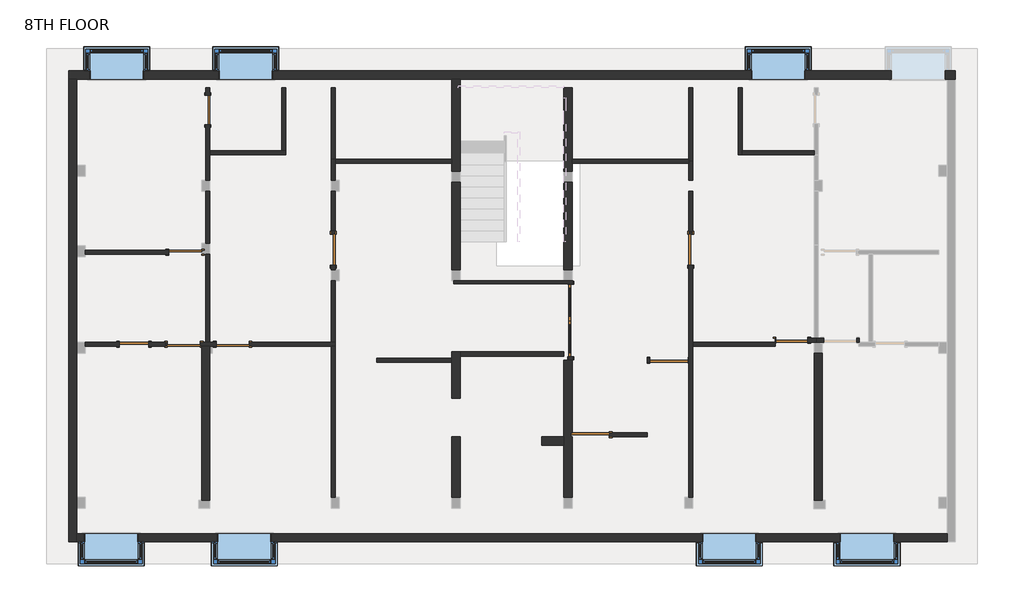
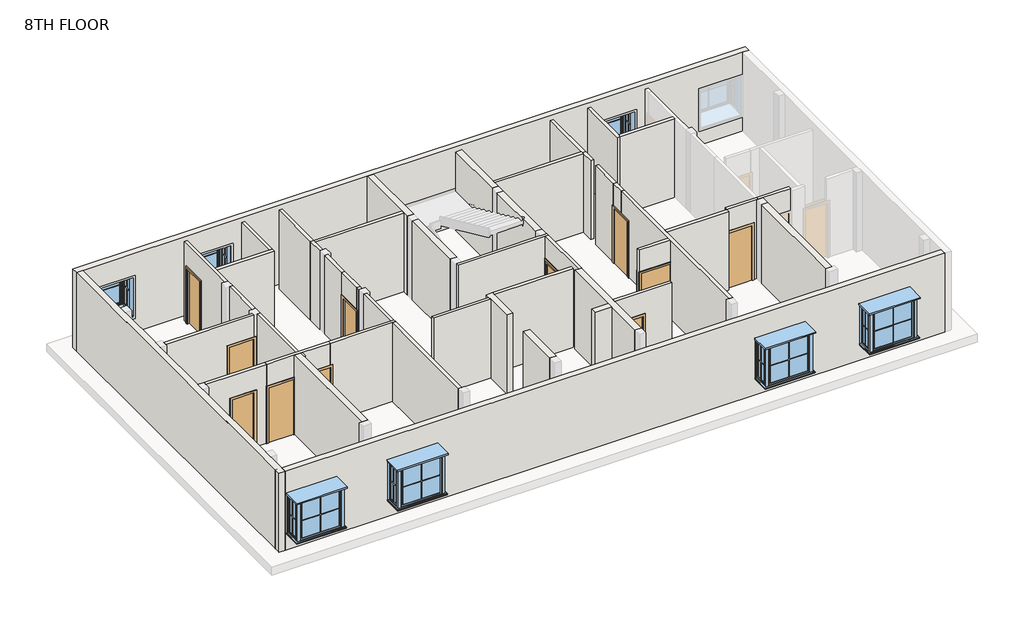
# One storey, part 1 of 2: 48 walls, 11 doors, 7 windows.
"""IFC4 building model written with IfcOpenShell, lengths in millimetres."""

from ifc_helpers import new_model, si_unit, frame, origin, place, context, project, spatial, polyline, outline, extrude, faceted_brep, transform, mapped, element, save
from components import door_04ab2522, m_door_single_panel_05506f71, door_07b5d71c, door_85b31ab1, door_1991e9a2, door_4c0a2014, door_82def9da, m_door_single_panel_3_x7_f8176753, m_door_single_panel_3_x7_ebb67e73, window_19bbd869

model = new_model("IFC4")

# Units and contexts
model_context = context("Model", 3, world=origin())
ifc_project = project(units=[si_unit("LENGTHUNIT", "METRE", prefix="MILLI")], contexts=[model_context])

# Site, building, storey
site = spatial("IfcSite", under=ifc_project)
building = spatial("IfcBuilding", under=site)
storey = spatial("IfcBuildingStorey", under=building, Name="8TH FLOOR", Elevation=28803.6)

# Doors
placement = place(None, origin())
door_shape = door_04ab2522(model_context)
element("IfcDoor", 1, ObjectType="M_Door-Double-Glass : 6'7\"X7'", at=placement, inside=storey, context=model_context, shape_type="MappedRepresentation", body=[
    mapped(door_shape, transform((1217.5394962, 1183.3817656, 28803.6), x_axis=(0.0, 1.0, 0.0), y_axis=(-1.0, 0.0, 0.0), z_axis=(0.0, 0.0, 1.0))),
])
m_door_single_panel_shape = m_door_single_panel_05506f71(model_context)
element("IfcDoor", 2, ObjectType="M_Door-Single-Panel", at=placement, inside=storey, context=model_context, shape_type="MappedRepresentation", body=[
    mapped(m_door_single_panel_shape, transform((1745.3012085, -1975.7432663, 28803.6), x_axis=(-1.0, 0.0, 0.0), y_axis=(0.0, -1.0, 0.0), z_axis=(0.0, 0.0, 1.0))),
])
element("IfcDoor", 3, ObjectType="M_Door-Single-Panel", at=placement, inside=storey, context=model_context, shape_type="MappedRepresentation", body=[
    mapped(m_door_single_panel_shape, transform((3933.4813133, 90.9578621, 28803.6), x_axis=(1.0, 0.0, 0.0), y_axis=(0.0, 1.0, 0.0), z_axis=(0.0, 0.0, 1.0))),
])
door_2_shape = door_07b5d71c(model_context)
element("IfcDoor", 4, ObjectType="M_Door-Single-Panel : 2'10\"X7' 2", at=placement, inside=storey, context=model_context, shape_type="MappedRepresentation", body=[
    mapped(door_2_shape, transform((-5360.3487995, 3142.9626891, 28803.6), x_axis=(0.0, -1.0, 0.0), y_axis=(1.0, 0.0, 0.0), z_axis=(0.0, 0.0, 1.0))),
])
door_3_shape = door_85b31ab1(model_context)
element("IfcDoor", 5, ObjectType="M_Door-Single-Panel : 2'10\"X7' 2", at=placement, inside=storey, context=model_context, shape_type="MappedRepresentation", body=[
    mapped(door_3_shape, transform((4532.9512082, 3142.9626891, 28803.6), x_axis=(0.0, -1.0, 0.0), y_axis=(1.0, 0.0, 0.0), z_axis=(0.0, 0.0, 1.0))),
])
door_4_shape = door_1991e9a2(model_context)
element("IfcDoor", 6, ObjectType="M_Door-Single-Panel : 2'11\"X7' 3", at=placement, inside=storey, context=model_context, shape_type="MappedRepresentation", body=[
    mapped(door_4_shape, transform((7330.1405552, 640.4567334, 28803.6), x_axis=(1.0, 0.0, 0.0), y_axis=(0.0, 1.0, 0.0), z_axis=(0.0, 0.0, 1.0))),
])
door_5_shape = door_4c0a2014(model_context)
element("IfcDoor", 7, ObjectType="M_Door-Single-Panel : 2'8\"X7'", at=placement, inside=storey, context=model_context, shape_type="MappedRepresentation", body=[
    mapped(door_5_shape, transform((-10873.4462614, 526.1567334, 28803.6), x_axis=(1.0, 0.0, 0.0), y_axis=(0.0, 1.0, 0.0), z_axis=(0.0, 0.0, 1.0))),
])
door_6_shape = door_82def9da(model_context)
element("IfcDoor", 8, ObjectType="M_Door-Single-Panel : 2'8\"X7'", at=placement, inside=storey, context=model_context, shape_type="MappedRepresentation", body=[
    mapped(door_6_shape, transform((-8827.4487992, 7008.6751452, 28803.6), x_axis=(0.0, 1.0, 0.0), y_axis=(-1.0, 0.0, 0.0), z_axis=(0.0, 0.0, 1.0))),
])
m_door_single_panel_3_x7_shape = m_door_single_panel_3_x7_f8176753(model_context)
element("IfcDoor", 9, ObjectType="M_Door-Single-Panel : 3'X7'", at=placement, inside=storey, context=model_context, shape_type="MappedRepresentation", body=[
    mapped(m_door_single_panel_3_x7_shape, transform((-9456.0987989, 3078.8567332, 28803.6), x_axis=(1.0, 0.0, 0.0), y_axis=(0.0, 1.0, 0.0), z_axis=(0.0, 0.0, 1.0))),
])
element("IfcDoor", 10, ObjectType="M_Door-Single-Panel : 3'X7'", at=placement, inside=storey, context=model_context, shape_type="MappedRepresentation", body=[
    mapped(m_door_single_panel_3_x7_shape, transform((-8144.8381465, 526.1567334, 28803.6), x_axis=(-1.0, 0.0, 0.0), y_axis=(0.0, -1.0, 0.0), z_axis=(0.0, 0.0, 1.0))),
])
m_door_single_panel_3_x7_2_shape = m_door_single_panel_3_x7_ebb67e73(model_context)
element("IfcDoor", 11, ObjectType="M_Door-Single-Panel : 3'X7'", at=placement, inside=storey, context=model_context, shape_type="MappedRepresentation", body=[
    mapped(m_door_single_panel_3_x7_2_shape, transform((-9494.1987992, 526.1567334, 28803.6), x_axis=(1.0, 0.0, 0.0), y_axis=(0.0, 1.0, 0.0), z_axis=(0.0, 0.0, 1.0))),
])

# Walls
element("IfcWall", 12, ObjectType="3.5\"", at=placement, inside=storey, context=model_context, shape_type="Brep", body=[
    faceted_brep([(-2020.2487998, 2196.2067742, 28803.6), (1158.0082462, 2196.2067742, 28803.6), (1272.3082462, 2196.2067742, 28803.6), (1272.3082462, 2196.2067742, 31851.6), (1158.0082462, 2196.2067742, 31851.6), (-2020.2487998, 2196.2067742, 31851.6), (-2020.2487998, 2285.1067742, 28803.6), (-2020.2487998, 2285.1067742, 31851.6), (-1845.5417538, 2285.1067742, 31851.6), (1024.6582462, 2285.1067742, 31851.6), (1253.2582462, 2285.1067742, 31851.6), (1272.3082462, 2285.1067742, 31851.6), (1272.3082462, 2285.1067742, 28803.6), (1253.2582462, 2285.1067742, 28803.6), (1024.6582462, 2285.1067742, 28803.6), (-1845.5417538, 2285.1067742, 28803.6)], [[[0, 1, 2, 3, 4, 5]], [[6, 7, 8, 9, 10, 11, 12, 13, 14, 15]], [[2, 1, 0, 6, 15, 14, 13, 12]], [[5, 4, 3, 11, 10, 9, 8, 7]], [[0, 5, 7, 6]], [[3, 2, 12, 11]]]),
])
element("IfcWall", 13, ObjectType="4.5\"", at=placement, inside=storey, context=model_context, shape_type="SweptSolid", body=[
    extrude(outline(polyline([(3132.0737955, 31851.6), (3628.3344162, 31851.6), (3628.3344162, 28803.6), (3574.7626891, 28803.6), (3574.7626891, 30937.2), (3132.0737955, 30937.2), (3132.0737955, 31851.6)])), frame((4475.8012082, 0.0, 0.0), z_axis=(1.0, 0.0, 0.0), x_axis=(0.0, 1.0, 0.0)), (0.0, 0.0, 1.0), 114.3),
])
element("IfcWall", 14, ObjectType="4.5\"", at=placement, inside=storey, context=model_context, shape_type="SweptSolid", body=[
    extrude(outline(polyline([(2711.1626891, 31851.6), (3671.8272228, 31851.6), (3671.8272228, 28803.6), (3574.7626891, 28803.6), (3574.7626891, 30937.2), (2711.1626891, 30937.2), (2711.1626891, 31851.6)])), frame((-5417.4987995, 0.0, 0.0), z_axis=(1.0, 0.0, 0.0), x_axis=(0.0, 1.0, 0.0)), (0.0, 0.0, 1.0), 114.3),
])
element("IfcWall", 15, ObjectType="4.5\"", at=placement, inside=storey, context=model_context, shape_type="Brep", body=[
    faceted_brep([(-7690.1644155, 469.0067334, 31851.6), (-8713.148796, 469.0067334, 31851.6), (-8771.750543, 469.0067334, 31851.6), (-9000.350543, 469.0067334, 31851.6), (-10009.8462614, 469.0067334, 31851.6), (-10009.8462614, 469.0067334, 28803.6), (-9951.3987992, 469.0067334, 28803.6), (-9951.3987992, 469.0067334, 30937.2), (-9036.9987992, 469.0067334, 30937.2), (-9036.9987992, 469.0067334, 28803.6), (-9000.350543, 469.0067334, 28803.6), (-8771.750543, 469.0067334, 28803.6), (-8713.148796, 469.0067334, 28803.6), (-8602.0381465, 469.0067334, 28803.6), (-8602.0381465, 469.0067334, 30937.2), (-7690.1644155, 469.0067334, 30937.2), (-10009.8462614, 583.3067334, 31851.6), (-7690.1644155, 583.3067334, 31851.6), (-7690.1644155, 583.3067334, 30937.2), (-8602.0381465, 583.3067334, 30937.2), (-8602.0381465, 583.3067334, 28803.6), (-9036.9987992, 583.3067334, 28803.6), (-9036.9987992, 583.3067334, 30937.2), (-9951.3987992, 583.3067334, 30937.2), (-9951.3987992, 583.3067334, 28803.6), (-10009.8462614, 583.3067334, 28803.6)], [[[0, 1, 2, 3, 4, 5, 6, 7, 8, 9, 10, 11, 12, 13, 14, 15]], [[16, 17, 18, 19, 20, 21, 22, 23, 24, 25]], [[5, 25, 24, 6]], [[9, 21, 20, 13, 12, 11, 10]], [[17, 0, 15, 18]], [[4, 3, 2, 1, 0, 17, 16]], [[5, 4, 16, 25]], [[8, 22, 21, 9]], [[7, 23, 22, 8]], [[23, 7, 6, 24]], [[19, 14, 13, 20]], [[14, 19, 18, 15]]]),
])
element("IfcWall", 16, ObjectType="4.5\"", at=placement, inside=storey, context=model_context, shape_type="Brep", body=[
    faceted_brep([(8000.0512079, 583.3067334, 28803.6), (8000.0512079, 583.3067334, 31851.6), (7942.9012047, 583.3067334, 31851.6), (6862.7668241, 583.3067334, 31851.6), (6862.7668241, 583.3067334, 28803.6), (6885.6405552, 583.3067334, 28803.6), (6885.6405552, 583.3067334, 30937.2), (7774.6405552, 583.3067334, 30937.2), (7774.6405552, 583.3067334, 28803.6), (7942.9012047, 583.3067334, 28803.6), (8000.0512079, 697.6067334, 31851.6), (8000.0512079, 697.6067334, 28803.6), (7942.9012079, 697.6067334, 28803.6), (7774.6405552, 697.6067334, 28803.6), (7774.6405552, 697.6067334, 30937.2), (6885.6405552, 697.6067334, 30937.2), (6885.6405552, 697.6067334, 28803.6), (6862.7668241, 697.6067334, 28803.6), (6862.7668241, 697.6067334, 31851.6), (7942.9012079, 697.6067334, 31851.6)], [[[0, 1, 2, 3, 4, 5, 6, 7, 8, 9]], [[10, 11, 12, 13, 14, 15, 16, 17, 18, 19]], [[4, 17, 16, 5]], [[11, 0, 9, 8, 13, 12]], [[1, 0, 11, 10]], [[3, 2, 1, 10, 19, 18]], [[4, 3, 18, 17]], [[7, 14, 13, 8]], [[14, 7, 6, 15]], [[15, 6, 5, 16]]]),
])
element("IfcWall", 17, ObjectType="4.5\"", at=placement, inside=storey, context=model_context, shape_type="Brep", body=[
    faceted_brep([(9187.5012047, 583.3067334, 28803.6), (9187.5012047, 583.3067334, 31851.6), (8171.5012047, 583.3067334, 31851.6), (8000.0512079, 583.3067334, 31851.6), (8000.0512079, 583.3067334, 28803.6), (8171.5012047, 583.3067334, 28803.6), (8209.6012079, 583.3067334, 28803.6), (8209.6012079, 583.3067334, 30937.2), (9124.0012079, 583.3067334, 30937.2), (9124.0012079, 583.3067334, 28803.6), (9187.5012047, 697.6067334, 31851.6), (9187.5012047, 697.6067334, 28803.6), (9124.0012079, 697.6067334, 28803.6), (9124.0012079, 697.6067334, 30937.2), (8209.6012079, 697.6067334, 30937.2), (8209.6012079, 697.6067334, 28803.6), (8057.2012079, 697.6067334, 28803.6), (8000.0512079, 697.6067334, 28803.6), (8000.0512079, 697.6067334, 31851.6), (8057.2012079, 697.6067334, 31851.6)], [[[0, 1, 2, 3, 4, 5, 6, 7, 8, 9]], [[10, 11, 12, 13, 14, 15, 16, 17, 18, 19]], [[11, 0, 9, 12]], [[4, 17, 16, 15, 6, 5]], [[1, 0, 11, 10]], [[3, 2, 1, 10, 19, 18]], [[4, 3, 18, 17]], [[7, 14, 13, 8]], [[8, 13, 12, 9]], [[14, 7, 6, 15]]]),
])
element("IfcWall", 18, ObjectType="4.5\"", at=placement, inside=storey, context=model_context, shape_type="SweptSolid", body=[
    extrude(outline(polyline([(28803.6, 3334.0114184), (31851.6, 3334.0114184), (31851.6, 1250.0012085), (30937.2, 1250.0012085), (30937.2, 2278.7012085), (28803.6, 2278.7012085), (28803.6, 3334.0114184)])), frame((0.0, -2032.8932663, 0.0), z_axis=(0.0, 1.0, 0.0), x_axis=(0.0, 0.0, 1.0)), (0.0, 0.0, 1.0), 114.3),
])
element("IfcWall", 19, ObjectType="4.5\"", at=placement, inside=storey, context=model_context, shape_type="SweptSolid", body=[
    extrude(outline(polyline([(30937.2, 4466.8813133), (28803.6, 4466.8813133), (28803.6, 4475.8012082), (31851.6, 4475.8012082), (31851.6, 3334.0114184), (28803.6, 3334.0114184), (28803.6, 3400.0813133), (30937.2, 3400.0813133), (30937.2, 4466.8813133)])), frame((0.0, 33.8078621, 0.0), z_axis=(0.0, 1.0, 0.0), x_axis=(0.0, 0.0, 1.0)), (0.0, 0.0, 1.0), 114.3),
])
element("IfcWall", 20, ObjectType="4.5\"", at=placement, inside=storey, context=model_context, shape_type="SweptSolid", body=[
    extrude(outline(polyline([(1021.4012085, 202.3067742), (-1848.7987998, 202.3067742), (-1848.7987998, 316.6067742), (1021.4012085, 316.6067742), (1021.4012085, 202.3067742)])), frame((0.0, 0.0, 28803.6), z_axis=(0.0, 0.0, 1.0), x_axis=(1.0, 0.0, 0.0)), (0.0, 0.0, 1.0), 3048.0),
])
element("IfcWall", 21, ObjectType="4.5\"", at=placement, inside=storey, context=model_context, shape_type="Brep", body=[
    faceted_brep([(1158.0082462, 2196.2067742, 28803.6), (1158.0082462, 2186.6817656, 28803.6), (1158.0082462, 2186.6817656, 30937.2), (1158.0082462, 180.0817656, 30937.2), (1158.0082462, 180.0817656, 28803.6), (1158.0082462, 90.9578621, 28803.6), (1158.0082462, 90.9578621, 31851.6), (1158.0082462, 2196.2067742, 31851.6), (1272.3082462, 2186.6817656, 30937.2), (1272.3082462, 2186.6817656, 28803.6), (1272.3082462, 2196.2067742, 28803.6), (1272.3082462, 2196.2067742, 31851.6), (1272.3082462, 90.9578621, 31851.6), (1272.3082462, 90.9578621, 28803.6), (1272.3082462, 180.0817656, 28803.6), (1272.3082462, 180.0817656, 30937.2), (1250.0012085, 90.9578621, 28803.6), (1250.0012085, 90.9578621, 31851.6)], [[[0, 1, 2, 3, 4, 5, 6, 7]], [[8, 9, 10, 11, 12, 13, 14, 15]], [[14, 13, 16, 5, 4]], [[10, 9, 1, 0]], [[6, 5, 16, 13, 12, 17]], [[7, 6, 17, 12, 11]], [[0, 7, 11, 10]], [[2, 1, 9, 8]], [[3, 2, 8, 15]], [[4, 3, 15, 14]]]),
])
element("IfcWall", 22, ObjectType="4.5\"", at=placement, inside=storey, context=model_context, shape_type="Brep", body=[
    faceted_brep([(1250.0012085, 5536.3067329, 28803.6), (4475.8012082, 5536.3067329, 28803.6), (4475.8012082, 5536.3067329, 31851.6), (1250.0012085, 5536.3067329, 31851.6), (1250.0012085, 5650.6067329, 28803.6), (1250.0012085, 5650.6067329, 31851.6), (4475.8012082, 5650.6067329, 31851.6), (4475.8012082, 5650.6067329, 28803.6), (4475.8012082, 5593.4567329, 28803.6), (4475.8012082, 5593.4567329, 31851.6)], [[[0, 1, 2, 3]], [[4, 5, 6, 7]], [[1, 0, 4, 7, 8]], [[3, 2, 9, 6, 5]], [[2, 1, 8, 7, 6, 9]], [[0, 3, 5, 4]]]),
])
element("IfcWall", 23, ObjectType="4.5\"", at=placement, inside=storey, context=model_context, shape_type="SweptSolid", body=[
    extrude(outline(polyline([(-5417.4987995, -3709.2932193), (-5417.4987995, 469.0067334), (-5303.1987995, 469.0067334), (-5303.1987995, -3709.2932193), (-5417.4987995, -3709.2932193)])), frame((0.0, 0.0, 28803.6), z_axis=(0.0, 0.0, 1.0), x_axis=(1.0, 0.0, 0.0)), (0.0, 0.0, 1.0), 3048.0),
])
element("IfcWall", 24, ObjectType="4.5\" 2", at=placement, inside=storey, context=model_context, shape_type="SweptSolid", body=[
    extrude(outline(polyline([(31851.6, -8998.8987989), (31851.6, -12224.6987989), (28803.6, -12224.6987989), (28803.6, -9913.2987989), (30937.2, -9913.2987989), (30937.2, -8998.8987989), (31851.6, -8998.8987989)])), frame((0.0, 3021.7067332, 0.0), z_axis=(0.0, 1.0, 0.0), x_axis=(0.0, 0.0, 1.0)), (0.0, 0.0, 1.0), 114.3),
])
element("IfcWall", 25, ObjectType="4.5\" 2", at=placement, inside=storey, context=model_context, shape_type="SweptSolid", body=[
    extrude(outline(polyline([(-8770.2987992, 4761.606733), (-8770.2987992, 3326.5067332), (-8884.5987992, 3326.5067332), (-8884.5987992, 4761.606733), (-8770.2987992, 4761.606733)])), frame((0.0, 0.0, 28803.6), z_axis=(0.0, 0.0, 1.0), x_axis=(1.0, 0.0, 0.0)), (0.0, 0.0, 1.0), 3048.0),
])
element("IfcWall", 26, ObjectType="4.5\" 2", at=placement, inside=storey, context=model_context, shape_type="Brep", body=[
    faceted_brep([(-8770.2987992, 7415.0751452, 30937.2), (-8770.2987992, 7415.0751452, 28803.6), (-8770.2987992, 7631.8067329, 28803.6), (-8770.2987992, 7631.8067329, 31851.6), (-8770.2987992, 5879.2067329, 31851.6), (-8770.2987992, 5764.9067329, 31851.6), (-8770.2987992, 5066.406733, 31851.6), (-8770.2987992, 5066.406733, 28803.6), (-8770.2987992, 5764.9067329, 28803.6), (-8770.2987992, 5879.2067329, 28803.6), (-8770.2987992, 6602.2751452, 28803.6), (-8770.2987992, 6602.2751452, 30937.2), (-8884.5987992, 7631.8067329, 28803.6), (-8884.5987992, 7415.0751452, 28803.6), (-8884.5987992, 7415.0751452, 30937.2), (-8884.5987992, 6602.2751452, 30937.2), (-8884.5987992, 6602.2751452, 28803.6), (-8884.5987992, 5066.406733, 28803.6), (-8884.5987992, 5066.406733, 31851.6), (-8884.5987992, 7631.8067329, 31851.6)], [[[0, 1, 2, 3, 4, 5, 6, 7, 8, 9, 10, 11]], [[12, 13, 14, 15, 16, 17, 18, 19]], [[2, 1, 13, 12]], [[10, 9, 8, 7, 17, 16]], [[3, 2, 12, 19]], [[6, 5, 4, 3, 19, 18]], [[7, 6, 18, 17]], [[14, 13, 1, 0]], [[15, 14, 0, 11]], [[16, 15, 11, 10]]]),
])
element("IfcWall", 27, ObjectType="4.5\" 2", at=placement, inside=storey, context=model_context, shape_type="Brep", body=[
    faceted_brep([(-8770.2987992, 5764.9067329, 28803.6), (-6674.7987994, 5764.9067329, 28803.6), (-6674.7987994, 5764.9067329, 31851.6), (-8770.2987992, 5764.9067329, 31851.6), (-8770.2987992, 5879.2067329, 28803.6), (-8770.2987992, 5879.2067329, 31851.6), (-6789.0987994, 5879.2067329, 31851.6), (-6674.7987994, 5879.2067329, 31851.6), (-6674.7987994, 5879.2067329, 28803.6), (-6789.0987994, 5879.2067329, 28803.6)], [[[0, 1, 2, 3]], [[4, 5, 6, 7, 8, 9]], [[1, 0, 4, 9, 8]], [[3, 2, 7, 6, 5]], [[0, 3, 5, 4]], [[2, 1, 8, 7]]]),
])
element("IfcWall", 28, ObjectType="4.5\" 2", at=placement, inside=storey, context=model_context, shape_type="SweptSolid", body=[
    extrude(outline(polyline([(-6674.7987994, 7631.8067329), (-6674.7987994, 5879.2067329), (-6789.0987994, 5879.2067329), (-6789.0987994, 7631.8067329), (-6674.7987994, 7631.8067329)])), frame((0.0, 0.0, 28803.6), z_axis=(0.0, 0.0, 1.0), x_axis=(1.0, 0.0, 0.0)), (0.0, 0.0, 1.0), 3048.0),
])
element("IfcWall", 29, ObjectType="4.5\" 2", at=placement, inside=storey, context=model_context, shape_type="SweptSolid", body=[
    extrude(outline(polyline([(30937.2, -10467.0462614), (28803.6, -10467.0462614), (28803.6, -10009.8462614), (31851.6, -10009.8462614), (31851.6, -12224.6987989), (28803.6, -12224.6987989), (28803.6, -11279.8462614), (30937.2, -11279.8462614), (30937.2, -10467.0462614)])), frame((0.0, 469.0067334, 0.0), z_axis=(0.0, 1.0, 0.0), x_axis=(0.0, 0.0, 1.0)), (0.0, 0.0, 1.0), 114.3),
])
element("IfcWall", 30, ObjectType="4.5\" 2", at=placement, inside=storey, context=model_context, shape_type="SweptSolid", body=[
    extrude(outline(polyline([(-8770.298796, 3021.7067332), (-8770.298796, 583.3067804), (-8884.598796, 583.3067804), (-8884.598796, 3021.7067332), (-8770.298796, 3021.7067332)])), frame((0.0, 0.0, 28803.6), z_axis=(0.0, 0.0, 1.0), x_axis=(1.0, 0.0, 0.0)), (0.0, 0.0, 1.0), 3048.0),
])
element("IfcWall", 31, ObjectType="4.5\" 2", at=placement, inside=storey, context=model_context, shape_type="Brep", body=[
    faceted_brep([(-5303.1987995, 469.0067334, 31851.6), (-5417.4987995, 469.0067334, 31851.6), (-7690.1644155, 469.0067334, 31851.6), (-7690.1644155, 469.0067334, 30937.2), (-7687.6381465, 469.0067334, 30937.2), (-7687.6381465, 469.0067334, 28803.6), (-5417.4987995, 469.0067334, 28803.6), (-5303.1987995, 469.0067334, 28803.6), (-7690.1644155, 583.3067334, 31851.6), (-5417.4987995, 583.3067334, 31851.6), (-5303.1987995, 583.3067334, 31851.6), (-5303.1987995, 583.3067334, 28803.6), (-5417.4987995, 583.3067334, 28803.6), (-7687.6381465, 583.3067334, 28803.6), (-7687.6381465, 583.3067334, 30937.2), (-7690.1644155, 583.3067334, 30937.2)], [[[0, 1, 2, 3, 4, 5, 6, 7]], [[8, 9, 10, 11, 12, 13, 14, 15]], [[11, 7, 6, 5, 13, 12]], [[2, 1, 0, 10, 9, 8]], [[2, 8, 15, 3]], [[0, 7, 11, 10]], [[14, 4, 3, 15]], [[4, 14, 13, 5]]]),
])
element("IfcWall", 32, ObjectType="4.5\" 2", at=placement, inside=storey, context=model_context, shape_type="SweptSolid", body=[
    extrude(outline(polyline([(-5303.1987995, 2285.1067802), (-5303.1987995, 583.3067334), (-5417.4987995, 583.3067334), (-5417.4987995, 2285.1067802), (-5303.1987995, 2285.1067802)])), frame((0.0, 0.0, 28803.6), z_axis=(0.0, 0.0, 1.0), x_axis=(1.0, 0.0, 0.0)), (0.0, 0.0, 1.0), 3048.0),
])
element("IfcWall", 33, ObjectType="4.5\" 2", at=placement, inside=storey, context=model_context, shape_type="Brep", body=[
    faceted_brep([(-5303.1987995, 2589.9067802, 28803.6), (-5303.1987995, 2711.1626891, 28803.6), (-5303.1987995, 2711.1626891, 30937.2), (-5303.1987995, 2711.1626891, 31851.6), (-5303.1987995, 2589.9067802, 31851.6), (-5417.4987995, 2589.9067802, 28803.6), (-5417.4987995, 2589.9067802, 31851.6), (-5417.4987995, 2711.1626891, 31851.6), (-5417.4987995, 2711.1626891, 30937.2), (-5417.4987995, 2711.1626891, 28803.6)], [[[0, 1, 2, 3, 4]], [[5, 6, 7, 8, 9]], [[1, 0, 5, 9]], [[3, 2, 1, 9, 8, 7]], [[4, 3, 7, 6]], [[0, 4, 6, 5]]]),
])
element("IfcWall", 34, ObjectType="4.5\" 2", at=placement, inside=storey, context=model_context, shape_type="SweptSolid", body=[
    extrude(outline(polyline([(-5303.1987995, 4761.606733), (-5303.1987995, 3671.8272228), (-5417.4987995, 3671.8272228), (-5417.4987995, 4761.606733), (-5303.1987995, 4761.606733)])), frame((0.0, 0.0, 28803.6), z_axis=(0.0, 0.0, 1.0), x_axis=(1.0, 0.0, 0.0)), (0.0, 0.0, 1.0), 3048.0),
])
element("IfcWall", 35, ObjectType="4.5\" 2", at=placement, inside=storey, context=model_context, shape_type="Brep", body=[
    faceted_brep([(-5303.1987995, 5066.406733, 28803.6), (-5303.1987995, 5536.3067329, 28803.6), (-5303.1987995, 5650.6067329, 28803.6), (-5303.1987995, 5650.6067329, 31851.6), (-5303.1987995, 5536.3067329, 31851.6), (-5303.1987995, 5066.406733, 31851.6), (-5417.4987995, 5066.406733, 28803.6), (-5417.4987995, 5066.406733, 31851.6), (-5417.4987995, 5650.6067329, 31851.6), (-5417.4987995, 5650.6067329, 28803.6)], [[[0, 1, 2, 3, 4, 5]], [[6, 7, 8, 9]], [[2, 1, 0, 6, 9]], [[5, 4, 3, 8, 7]], [[0, 5, 7, 6]], [[3, 2, 9, 8]]]),
])
element("IfcWall", 36, ObjectType="4.5\" 2", at=placement, inside=storey, context=model_context, shape_type="SweptSolid", body=[
    extrude(outline(polyline([(-2077.3987998, 5536.3067329), (-5303.1987995, 5536.3067329), (-5303.1987995, 5650.6067329), (-2077.3987998, 5650.6067329), (-2077.3987998, 5536.3067329)])), frame((0.0, 0.0, 28803.6), z_axis=(0.0, 0.0, 1.0), x_axis=(1.0, 0.0, 0.0)), (0.0, 0.0, 1.0), 3048.0),
])
element("IfcWall", 37, ObjectType="4.5\" 2", at=placement, inside=storey, context=model_context, shape_type="SweptSolid", body=[
    extrude(outline(polyline([(-5417.4987995, 5650.6067329), (-5417.4987995, 7631.8067329), (-5303.1987995, 7631.8067329), (-5303.1987995, 5650.6067329), (-5417.4987995, 5650.6067329)])), frame((0.0, 0.0, 28803.6), z_axis=(0.0, 0.0, 1.0), x_axis=(1.0, 0.0, 0.0)), (0.0, 0.0, 1.0), 3048.0),
])
element("IfcWall", 38, ObjectType="4.5\" 2", at=placement, inside=storey, context=model_context, shape_type="Brep", body=[
    faceted_brep([(4475.8012082, 5593.4567329, 28803.6), (4475.8012082, 5536.3067329, 28803.6), (4475.8012082, 5066.40678, 28803.6), (4475.8012082, 5066.40678, 31851.6), (4475.8012082, 5536.3067329, 31851.6), (4475.8012082, 5593.4567329, 31851.6), (4590.1012082, 5593.4567329, 28803.6), (4590.1012082, 5593.4567329, 31851.6), (4590.1012082, 5066.40678, 31851.6), (4590.1012082, 5066.40678, 28803.6)], [[[0, 1, 2, 3, 4, 5]], [[6, 7, 8, 9]], [[2, 1, 0, 6, 9]], [[3, 2, 9, 8]], [[5, 4, 3, 8, 7]], [[0, 5, 7, 6]]]),
])
element("IfcWall", 39, ObjectType="4.5\" 2", at=placement, inside=storey, context=model_context, shape_type="SweptSolid", body=[
    extrude(outline(polyline([(4475.8012082, 3628.3344162), (4475.8012082, 4761.606733), (4590.1012082, 4761.606733), (4590.1012082, 3628.3344162), (4475.8012082, 3628.3344162)])), frame((0.0, 0.0, 28803.6), z_axis=(0.0, 0.0, 1.0), x_axis=(1.0, 0.0, 0.0)), (0.0, 0.0, 1.0), 3048.0),
])
element("IfcWall", 40, ObjectType="4.5\" 2", at=placement, inside=storey, context=model_context, shape_type="Brep", body=[
    faceted_brep([(4475.8012082, -3709.2932193, 28803.6), (4475.8012082, -3709.2932193, 31851.6), (4475.8012082, 33.8078621, 31851.6), (4475.8012082, 148.1078621, 31851.6), (4475.8012082, 3132.0737955, 31851.6), (4475.8012082, 3132.0737955, 30937.2), (4475.8012082, 2711.1626891, 30937.2), (4475.8012082, 2711.1626891, 28803.6), (4475.8012082, 148.1078621, 28803.6), (4475.8012082, 33.8078621, 28803.6), (4590.1012082, -3709.2932193, 31851.6), (4590.1012082, -3709.2932193, 28803.6), (4590.1012082, 469.0067334, 28803.6), (4590.1012082, 583.3067334, 28803.6), (4590.1012082, 2711.1626891, 28803.6), (4590.1012082, 2711.1626891, 30937.2), (4590.1012082, 3132.0737955, 30937.2), (4590.1012082, 3132.0737955, 31851.6), (4590.1012082, 583.3067334, 31851.6), (4590.1012082, 469.0067334, 31851.6)], [[[0, 1, 2, 3, 4, 5, 6, 7, 8, 9]], [[10, 11, 12, 13, 14, 15, 16, 17, 18, 19]], [[11, 0, 9, 8, 7, 14, 13, 12]], [[1, 0, 11, 10]], [[4, 3, 2, 1, 10, 19, 18, 17]], [[4, 17, 16, 5]], [[6, 15, 14, 7]], [[15, 6, 5, 16]]]),
])
element("IfcWall", 41, ObjectType="4.5\" 2", at=placement, inside=storey, context=model_context, shape_type="SweptSolid", body=[
    extrude(outline(polyline([(6862.7668241, 469.0067334), (4590.1012082, 469.0067334), (4590.1012082, 583.3067334), (6862.7668241, 583.3067334), (6862.7668241, 469.0067334)])), frame((0.0, 0.0, 28803.6), z_axis=(0.0, 0.0, 1.0), x_axis=(1.0, 0.0, 0.0)), (0.0, 0.0, 1.0), 3048.0),
])
element("IfcWall", 42, ObjectType="4.5\" 2", at=placement, inside=storey, context=model_context, shape_type="Brep", body=[
    faceted_brep([(4590.1012082, 5593.4567329, 28803.6), (4590.1012082, 7631.8067329, 28803.6), (4590.1012082, 7631.8067329, 31851.6), (4590.1012082, 5593.4567329, 31851.6), (4475.8012082, 5593.4567329, 28803.6), (4475.8012082, 5593.4567329, 31851.6), (4475.8012082, 5650.6067329, 31851.6), (4475.8012082, 7631.8067329, 31851.6), (4475.8012082, 7631.8067329, 28803.6), (4475.8012082, 5650.6067329, 28803.6)], [[[0, 1, 2, 3]], [[4, 5, 6, 7, 8, 9]], [[1, 0, 4, 9, 8]], [[2, 1, 8, 7]], [[3, 2, 7, 6, 5]], [[0, 3, 5, 4]]]),
])
element("IfcWall", 43, ObjectType="4.5\" 2", at=placement, inside=storey, context=model_context, shape_type="Brep", body=[
    faceted_brep([(5847.401208, 7631.8067329, 28803.6), (5847.401208, 5764.9067329, 28803.6), (5847.401208, 5764.9067329, 31851.6), (5847.401208, 7631.8067329, 31851.6), (5961.701208, 7631.8067329, 28803.6), (5961.701208, 7631.8067329, 31851.6), (5961.701208, 5879.2067329, 31851.6), (5961.701208, 5764.9067329, 31851.6), (5961.701208, 5764.9067329, 28803.6), (5961.701208, 5879.2067329, 28803.6)], [[[0, 1, 2, 3]], [[4, 5, 6, 7, 8, 9]], [[1, 0, 4, 9, 8]], [[3, 2, 7, 6, 5]], [[0, 3, 5, 4]], [[2, 1, 8, 7]]]),
])
element("IfcWall", 44, ObjectType="4.5\" 2", at=placement, inside=storey, context=model_context, shape_type="SweptSolid", body=[
    extrude(outline(polyline([(7942.9012079, 5764.9067329), (5961.701208, 5764.9067329), (5961.701208, 5879.2067329), (7942.9012079, 5879.2067329), (7942.9012079, 5764.9067329)])), frame((0.0, 0.0, 28803.6), z_axis=(0.0, 0.0, 1.0), x_axis=(1.0, 0.0, 0.0)), (0.0, 0.0, 1.0), 3048.0),
])
element("IfcWall", 45, ObjectType="4.5\" 2", at=placement, inside=storey, context=model_context, shape_type="SweptSolid", body=[
    extrude(outline(polyline([(-2077.3987998, 33.8078621), (-4161.4090098, 33.8078621), (-4161.4090098, 148.1078621), (-2077.3987998, 148.1078621), (-2077.3987998, 33.8078621)])), frame((0.0, 0.0, 28803.6), z_axis=(0.0, 0.0, 1.0), x_axis=(1.0, 0.0, 0.0)), (0.0, 0.0, 1.0), 3048.0),
])
element("IfcWall", 46, ObjectType="9\"", at=placement, inside=storey, context=model_context, shape_type="Brep", body=[
    faceted_brep([(-12681.8987957, 7860.4067329, 28803.6), (-12453.2987957, 7860.4067329, 28803.6), (-2074.1417538, 7860.4067329, 28803.6), (-1845.5417538, 7860.4067329, 28803.6), (11625.9012075, 7860.4067329, 28803.6), (11854.5012075, 7860.4067329, 28803.6), (11854.5012075, 7860.4067329, 31851.6), (11625.9012075, 7860.4067329, 31851.6), (-1845.5417538, 7860.4067329, 31851.6), (-2074.1417538, 7860.4067329, 31851.6), (-12453.2987957, 7860.4067329, 31851.6), (-12681.8987957, 7860.4067329, 31851.6), (11575.8012075, 7860.4067329, 30954.4), (11575.8012075, 7860.4067329, 29403.6), (10075.8012075, 7860.4067329, 29403.6), (10075.8012075, 7860.4067329, 30954.4), (7702.301208, 7860.4067329, 30954.4), (7702.301208, 7860.4067329, 29403.6), (6202.301208, 7860.4067329, 29403.6), (6202.301208, 7860.4067329, 30954.4), (-7029.6987993, 7860.4067329, 30954.4), (-7029.6987993, 7860.4067329, 29403.6), (-8529.6987993, 7860.4067329, 29403.6), (-8529.6987993, 7860.4067329, 30954.4), (-10598.3987957, 7860.4067329, 30954.4), (-10598.3987957, 7860.4067329, 29403.6), (-12098.3987957, 7860.4067329, 29403.6), (-12098.3987957, 7860.4067329, 30954.4), (-12681.8987957, 8089.0067329, 28803.6), (-12681.8987957, 8089.0067329, 31851.6), (11854.5012075, 8089.0067329, 31851.6), (11854.5012075, 8089.0067329, 28803.6), (11575.8012075, 8089.0067329, 30954.4), (10075.8012075, 8089.0067329, 30954.4), (10075.8012075, 8089.0067329, 29403.6), (11575.8012075, 8089.0067329, 29403.6), (7702.301208, 8089.0067329, 30954.4), (6202.301208, 8089.0067329, 30954.4), (6202.301208, 8089.0067329, 29403.6), (7702.301208, 8089.0067329, 29403.6), (-7029.6987993, 8089.0067329, 30954.4), (-8529.6987993, 8089.0067329, 30954.4), (-8529.6987993, 8089.0067329, 29403.6), (-7029.6987993, 8089.0067329, 29403.6), (-10598.3987957, 8089.0067329, 30954.4), (-12098.3987957, 8089.0067329, 30954.4), (-12098.3987957, 8089.0067329, 29403.6), (-10598.3987957, 8089.0067329, 29403.6)], [[[0, 1, 2, 3, 4, 5, 6, 7, 8, 9, 10, 11], [12, 13, 14, 15], [16, 17, 18, 19], [20, 21, 22, 23], [24, 25, 26, 27]], [[28, 29, 30, 31], [32, 33, 34, 35], [36, 37, 38, 39], [40, 41, 42, 43], [44, 45, 46, 47]], [[5, 4, 3, 2, 1, 0, 28, 31]], [[11, 10, 9, 8, 7, 6, 30, 29]], [[6, 5, 31, 30]], [[0, 11, 29, 28]], [[13, 12, 32, 35]], [[14, 13, 35, 34]], [[15, 14, 34, 33]], [[12, 15, 33, 32]], [[17, 16, 36, 39]], [[18, 17, 39, 38]], [[19, 18, 38, 37]], [[16, 19, 37, 36]], [[21, 20, 40, 43]], [[22, 21, 43, 42]], [[23, 22, 42, 41]], [[20, 23, 41, 40]], [[25, 24, 44, 47]], [[26, 25, 47, 46]], [[27, 26, 46, 45]], [[24, 27, 45, 44]]]),
])
element("IfcWall", 47, ObjectType="9\"", at=placement, inside=storey, context=model_context, shape_type="Brep", body=[
    faceted_brep([(-12453.2987957, -4941.1932661, 28803.6), (-12453.2987957, -4712.5932661, 28803.6), (-12453.2987957, -4014.0932671, 28803.6), (-12453.2987957, -3709.2932671, 28803.6), (-12453.2987957, 278.5067334, 28803.6), (-12453.2987957, 583.3067334, 28803.6), (-12453.2987957, 2951.8567332, 28803.6), (-12453.2987957, 3256.6567332, 28803.6), (-12453.2987957, 5174.3567339, 28803.6), (-12453.2987957, 5479.1567339, 28803.6), (-12453.2987957, 7860.4067329, 28803.6), (-12453.2987957, 7860.4067329, 31851.6), (-12453.2987957, 5479.1567339, 31851.6), (-12453.2987957, 5174.3567339, 31851.6), (-12453.2987957, 3256.6567332, 31851.6), (-12453.2987957, 2951.8567332, 31851.6), (-12453.2987957, 583.3067334, 31851.6), (-12453.2987957, 278.5067334, 31851.6), (-12453.2987957, -3709.2932671, 31851.6), (-12453.2987957, -4014.0932671, 31851.6), (-12453.2987957, -4712.5932661, 31851.6), (-12453.2987957, -4941.1932661, 31851.6), (-12681.8987957, -4941.1932661, 28803.6), (-12681.8987957, -4941.1932661, 31851.6), (-12681.8987957, 7860.4067329, 31851.6), (-12681.8987957, 7860.4067329, 28803.6)], [[[0, 1, 2, 3, 4, 5, 6, 7, 8, 9, 10, 11, 12, 13, 14, 15, 16, 17, 18, 19, 20, 21]], [[22, 23, 24, 25]], [[10, 9, 8, 7, 6, 5, 4, 3, 2, 1, 0, 22, 25]], [[21, 20, 19, 18, 17, 16, 15, 14, 13, 12, 11, 24, 23]], [[11, 10, 25, 24]], [[0, 21, 23, 22]]]),
])
element("IfcWall", 48, ObjectType="9\"", at=placement, inside=storey, context=model_context, shape_type="Brep", body=[
    faceted_brep([(-12453.2987957, -4712.5932661, 28803.6), (-12453.2987957, -4014.0932671, 28803.6), (-12453.2987957, -3709.2932671, 28803.6), (-12453.2987957, 278.5067334, 28803.6), (-12453.2987957, 583.3067334, 28803.6), (-12453.2987957, 2951.8567332, 28803.6), (-12453.2987957, 3256.6567332, 28803.6), (-12453.2987957, 5174.3567339, 28803.6), (-12453.2987957, 5479.1567339, 28803.6), (-12453.2987957, 7860.4067329, 28803.6), (-12453.2987957, 7860.4067329, 31851.6), (-12453.2987957, 5479.1567339, 31851.6), (-12453.2987957, 5174.3567339, 31851.6), (-12453.2987957, 3256.6567332, 31851.6), (-12453.2987957, 2951.8567332, 31851.6), (-12453.2987957, 583.3067334, 31851.6), (-12453.2987957, 278.5067334, 31851.6), (-12453.2987957, -3709.2932671, 31851.6), (-12453.2987957, -4014.0932671, 31851.6), (-12453.2987957, -4712.5932661, 31851.6), (-12681.8987957, -4712.5932661, 28803.6), (-12681.8987957, -4712.5932661, 31851.6), (-12681.8987957, 7860.4067329, 31851.6), (-12681.8987957, 7860.4067329, 28803.6)], [[[0, 1, 2, 3, 4, 5, 6, 7, 8, 9, 10, 11, 12, 13, 14, 15, 16, 17, 18, 19]], [[20, 21, 22, 23]], [[9, 8, 7, 6, 5, 4, 3, 2, 1, 0, 20, 23]], [[19, 18, 17, 16, 15, 14, 13, 12, 11, 10, 22, 21]], [[10, 9, 23, 22]], [[0, 19, 21, 20]]]),
])
element("IfcWall", 49, ObjectType="9\"", at=placement, inside=storey, context=model_context, shape_type="Brep", body=[
    faceted_brep([(-9000.350543, 469.0067334, 28803.6), (-9000.350543, -3785.4932196, 28803.6), (-9000.350543, -3785.4932196, 31851.6), (-9000.350543, 469.0067334, 31851.6), (-8771.750543, 469.0067334, 28803.6), (-8771.750543, 469.0067334, 31851.6), (-8771.750543, 278.5067334, 31851.6), (-8771.750543, -3785.4932196, 31851.6), (-8771.750543, -3785.4932196, 28803.6), (-8771.750543, 278.5067334, 28803.6)], [[[0, 1, 2, 3]], [[4, 5, 6, 7, 8, 9]], [[1, 0, 4, 9, 8]], [[2, 1, 8, 7]], [[3, 2, 7, 6, 5]], [[0, 3, 5, 4]]]),
])
element("IfcWall", 50, ObjectType="9\"", at=placement, inside=storey, context=model_context, shape_type="Brep", body=[
    faceted_brep([(-2077.3987998, 316.6067742, 28803.6), (-2077.3987998, 148.1078621, 28803.6), (-2077.3987998, 33.8078621, 28803.6), (-2077.3987998, -972.2341552, 28803.6), (-2077.3987998, -972.2341552, 31851.6), (-2077.3987998, 33.8078621, 31851.6), (-2077.3987998, 148.1078621, 31851.6), (-2077.3987998, 316.6067742, 31851.6), (-1848.7987998, 316.6067742, 28803.6), (-1848.7987998, 316.6067742, 31851.6), (-1848.7987998, 202.3067742, 31851.6), (-1848.7987998, -972.2341552, 31851.6), (-1848.7987998, -972.2341552, 28803.6), (-1848.7987998, 202.3067742, 28803.6)], [[[0, 1, 2, 3, 4, 5, 6, 7]], [[8, 9, 10, 11, 12, 13]], [[3, 2, 1, 0, 8, 13, 12]], [[4, 3, 12, 11]], [[7, 6, 5, 4, 11, 10, 9]], [[0, 7, 9, 8]]]),
])
element("IfcWall", 51, ObjectType="9\"", at=placement, inside=storey, context=model_context, shape_type="SweptSolid", body=[
    extrude(outline(polyline([(-2077.3987998, -3709.2932663), (-2077.3987998, -2032.8932663), (-1848.7987998, -2032.8932663), (-1848.7987998, -3709.2932663), (-2077.3987998, -3709.2932663)])), frame((0.0, 0.0, 28803.6), z_axis=(0.0, 0.0, 1.0), x_axis=(1.0, 0.0, 0.0)), (0.0, 0.0, 1.0), 3048.0),
])
element("IfcWall", 52, ObjectType="9\"", at=placement, inside=storey, context=model_context, shape_type="SweptSolid", body=[
    extrude(outline(polyline([(1021.4012085, -2261.4932663), (412.152227, -2261.4932663), (412.152227, -2032.8932663), (1021.4012085, -2032.8932663), (1021.4012085, -2261.4932663)])), frame((0.0, 0.0, 28803.6), z_axis=(0.0, 0.0, 1.0), x_axis=(1.0, 0.0, 0.0)), (0.0, 0.0, 1.0), 3048.0),
])
element("IfcWall", 53, ObjectType="9\"", at=placement, inside=storey, context=model_context, shape_type="Brep", body=[
    faceted_brep([(1021.4012085, 90.9578621, 28803.6), (1021.4012085, -2032.8932663, 28803.6), (1021.4012085, -2261.4932663, 28803.6), (1021.4012085, -3709.2932193, 28803.6), (1021.4012085, -3709.2932193, 31851.6), (1021.4012085, -2261.4932663, 31851.6), (1021.4012085, -2032.8932663, 31851.6), (1021.4012085, 90.9578621, 31851.6), (1250.0012085, -3709.2932193, 31851.6), (1250.0012085, -3709.2932193, 28803.6), (1250.0012085, -2032.8932663, 28803.6), (1250.0012085, -2032.8932663, 30937.2), (1250.0012085, -1918.5932663, 30937.2), (1250.0012085, -1918.5932663, 28803.6), (1250.0012085, 90.9578621, 28803.6), (1250.0012085, 90.9578621, 31851.6), (1250.0012085, -1918.5932663, 31851.6), (1250.0012085, -2032.8932663, 31851.6), (1158.0082462, 90.9578621, 28803.6), (1211.9012085, -1918.5932663, 28803.6), (1211.9012085, -2032.8932663, 28803.6), (1158.0082462, 90.9578621, 31851.6), (1211.9012085, -1918.5932663, 30937.2), (1211.9012085, -2032.8932663, 30937.2)], [[[0, 1, 2, 3, 4, 5, 6, 7]], [[8, 9, 10, 11, 12, 13, 14, 15, 16, 17]], [[3, 2, 1, 0, 18, 14, 13, 19, 20, 10, 9]], [[4, 3, 9, 8]], [[7, 6, 5, 4, 8, 17, 16, 15, 21]], [[0, 7, 21, 15, 14, 18]], [[22, 19, 13, 12]], [[20, 23, 11, 10]], [[19, 22, 23, 20]], [[23, 22, 12, 11]]]),
])
element("IfcWall", 54, ObjectType="9\"", at=placement, inside=storey, context=model_context, shape_type="SweptSolid", body=[
    extrude(outline(polyline([(-2074.1417538, 5320.4067329), (-2074.1417538, 7860.4067329), (-1845.5417538, 7860.4067329), (-1845.5417538, 5320.4067329), (-2074.1417538, 5320.4067329)])), frame((0.0, 0.0, 28803.6), z_axis=(0.0, 0.0, 1.0), x_axis=(1.0, 0.0, 0.0)), (0.0, 0.0, 1.0), 3048.0),
])
element("IfcWall", 55, ObjectType="9\"", at=placement, inside=storey, context=model_context, shape_type="SweptSolid", body=[
    extrude(outline(polyline([(-2074.1417538, 2589.906774), (-2074.1417538, 5015.606774), (-1845.5417538, 5015.606774), (-1845.5417538, 2589.906774), (-2074.1417538, 2589.906774)])), frame((0.0, 0.0, 28803.6), z_axis=(0.0, 0.0, 1.0), x_axis=(1.0, 0.0, 0.0)), (0.0, 0.0, 1.0), 3048.0),
])
element("IfcWall", 56, ObjectType="9\"", at=placement, inside=storey, context=model_context, shape_type="Brep", body=[
    faceted_brep([(1021.4012085, 7631.8067329, 28803.6), (1021.4012085, 5320.4067329, 28803.6), (1021.4012085, 5320.4067329, 31851.6), (1021.4012085, 7631.8067329, 31851.6), (1250.0012085, 7631.8067329, 28803.6), (1250.0012085, 7631.8067329, 31851.6), (1250.0012085, 5650.6067329, 31851.6), (1250.0012085, 5536.3067329, 31851.6), (1250.0012085, 5320.4067329, 31851.6), (1250.0012085, 5320.4067329, 28803.6), (1250.0012085, 5536.3067329, 28803.6), (1250.0012085, 5650.6067329, 28803.6)], [[[0, 1, 2, 3]], [[4, 5, 6, 7, 8, 9, 10, 11]], [[1, 0, 4, 11, 10, 9]], [[2, 1, 9, 8]], [[3, 2, 8, 7, 6, 5]], [[0, 3, 5, 4]]]),
])
element("IfcWall", 57, ObjectType="9\"", at=placement, inside=storey, context=model_context, shape_type="Brep", body=[
    faceted_brep([(1021.4012085, 5015.6067329, 28803.6), (1021.4012085, 2589.9067742, 28803.6), (1021.4012085, 2589.9067742, 31851.6), (1021.4012085, 5015.6067329, 31851.6), (1250.0012085, 5015.6067329, 28803.6), (1250.0012085, 5015.6067329, 31851.6), (1250.0012085, 2589.9067742, 31851.6), (1250.0012085, 2589.9067742, 28803.6), (1024.6582462, 2589.9067742, 28803.6), (1024.6582462, 2589.9067742, 31851.6)], [[[0, 1, 2, 3]], [[4, 5, 6, 7]], [[1, 0, 4, 7, 8]], [[2, 1, 8, 7, 6, 9]], [[3, 2, 9, 6, 5]], [[0, 3, 5, 4]]]),
])
element("IfcWall", 58, ObjectType="9\"", at=placement, inside=storey, context=model_context, shape_type="SweptSolid", body=[
    extrude(outline(polyline([(7942.9012047, -3785.4932666), (7942.9012047, 278.5067334), (8171.5012047, 278.5067334), (8171.5012047, -3785.4932666), (7942.9012047, -3785.4932666)])), frame((0.0, 0.0, 28803.6), z_axis=(0.0, 0.0, 1.0), x_axis=(1.0, 0.0, 0.0)), (0.0, 0.0, 1.0), 3048.0),
])
element("IfcWall", 59, ObjectType="9\" 2", at=placement, inside=storey, context=model_context, shape_type="SweptSolid", body=[
    extrude(outline(polyline([(28803.6, -12453.2987957), (28803.6, 11625.9012075), (31851.6, 11625.9012075), (31851.6, -12453.2987957), (28803.6, -12453.2987957)]), holes=[polyline([(30954.4, 8658.6146942), (30954.4, 10158.6146942), (29403.6, 10158.6146942), (29403.6, 8658.6146942), (30954.4, 8658.6146942)]), polyline([(30954.4, 4849.7512082), (30954.4, 6349.7512082), (29403.6, 6349.7512082), (29403.6, 4849.7512082), (30954.4, 4849.7512082)]), polyline([(30954.4, -8569.250543), (30954.4, -7069.250543), (29403.6, -7069.250543), (29403.6, -8569.250543), (30954.4, -8569.250543)]), polyline([(30954.4, -12250.7987957), (30954.4, -10750.7987957), (29403.6, -10750.7987957), (29403.6, -12250.7987957), (30954.4, -12250.7987957)])]), frame((0.0, -4941.1932661, 0.0), z_axis=(0.0, 1.0, 0.0), x_axis=(0.0, 0.0, 1.0)), (0.0, 0.0, 1.0), 228.6),
])

# Windows
window_shape = window_19bbd869(model_context)
element("IfcWindow", 60, ObjectType="4'.8\"x3'.8\"", at=placement, inside=storey, context=model_context, shape_type="MappedRepresentation", body=[
    mapped(window_shape, transform((-11500.7987957, -4826.8932661, 28803.6), x_axis=(-1.0, 0.0, 0.0), y_axis=(0.0, -1.0, 0.0), z_axis=(0.0, 0.0, 1.0))),
])
element("IfcWindow", 61, ObjectType="4'.8\"x3'.8\"", at=placement, inside=storey, context=model_context, shape_type="MappedRepresentation", body=[
    mapped(window_shape, transform((-7819.250543, -4826.8932661, 28803.6), x_axis=(-1.0, 0.0, 0.0), y_axis=(0.0, -1.0, 0.0), z_axis=(0.0, 0.0, 1.0))),
])
element("IfcWindow", 62, ObjectType="4'.8\"x3'.8\"", at=placement, inside=storey, context=model_context, shape_type="MappedRepresentation", body=[
    mapped(window_shape, transform((5599.7512082, -4826.8932661, 28803.6), x_axis=(-1.0, 0.0, 0.0), y_axis=(0.0, -1.0, 0.0), z_axis=(0.0, 0.0, 1.0))),
])
element("IfcWindow", 63, ObjectType="4'.8\"x3'.8\"", at=placement, inside=storey, context=model_context, shape_type="MappedRepresentation", body=[
    mapped(window_shape, transform((9408.6146942, -4826.8932661, 28803.6), x_axis=(-1.0, 0.0, 0.0), y_axis=(0.0, -1.0, 0.0), z_axis=(0.0, 0.0, 1.0))),
])
element("IfcWindow", 64, ObjectType="4'.8\"x3'.8\"", at=placement, inside=storey, context=model_context, shape_type="MappedRepresentation", body=[
    mapped(window_shape, transform((-11348.3987957, 7974.7067329, 28803.6), x_axis=(1.0, 0.0, 0.0), y_axis=(0.0, 1.0, 0.0), z_axis=(0.0, 0.0, 1.0))),
])
element("IfcWindow", 65, ObjectType="4'.8\"x3'.8\"", at=placement, inside=storey, context=model_context, shape_type="MappedRepresentation", body=[
    mapped(window_shape, transform((-7779.6987993, 7974.7067329, 28803.6), x_axis=(1.0, 0.0, 0.0), y_axis=(0.0, 1.0, 0.0), z_axis=(0.0, 0.0, 1.0))),
])
element("IfcWindow", 66, ObjectType="4'.8\"x3'.8\"", at=placement, inside=storey, context=model_context, shape_type="MappedRepresentation", body=[
    mapped(window_shape, transform((6952.301208, 7974.7067329, 28803.6), x_axis=(1.0, 0.0, 0.0), y_axis=(0.0, 1.0, 0.0), z_axis=(0.0, 0.0, 1.0))),
])

save(model, "model.ifc")

# Revit data of these elements
# Type "M_Door-Double-Glass : 6'7\"X7'"
#   Type Mark = "16"
#   Construction Type Id = "opn-d45"
#   Assembly Code = "C1020"
#   Analytic Construction = "Wood frame, double glass door "
#   W = 3' - 3 1/2"
#   Thickness = 0' - 1.9685"
#   Thermal Resistance (R) = 1.8150 (h·ft²·°F)/BTU
#   Swing Angle [instance default] = 90.00°
#   Heat Transfer Coefficient (U) = 0.5510 BTU/(h·ft²·°F)
#   Height = 7' - 0"
#   Bottom Rail = 0' - 3.93701"
#   Top Rail = 0' - 3.93701"
#   Stiles = 0' - 3.93701"
#   Trim Projection = 0' - 0.98425"
#   Trim Width = 0' - 3.14961"
#   Width = 6' - 7"
#   Define Thermal Properties by = 1
#   Glazing = Glass
#   Panel Material = Wood - Birch - Solid Stained Light Low Gloss
#   Trim Material = Paint - Sienna
#   Visual Light Transmittance = 0
#   Solar Heat Gain Coefficient = 0
#   Function = (empty or 0)
#   Wall Closure = (empty or 0)
# Type "M_Door-Single-Panel"
#   Type Mark = "14"
#   Construction Type Id = "DOOR"
#   Assembly Code = "C1020300"
#   Analytic Construction = "Wooden"
#   Thickness = 0' - 1.9685"
#   Thermal Resistance (R) = 2.5876 (h·ft²·°F)/BTU
#   Swing Angle [instance default] = 90.00°
#   Heat Transfer Coefficient (U) = 0.3865 BTU/(h·ft²·°F)
#   Height = 7' - 0"
#   Trim Projection Ext = 0' - 0.98425"
#   Trim Projection Int = 0' - 0.98425"
#   Trim Width = 0' - 3.14961"
#   Width = 3' - 6"
#   Define Thermal Properties by = 1
#   Panel Material = Wood - Birch - Solid Stained Light Low Gloss
#   Trim Material = Paint - Sienna
#   Visual Light Transmittance = 0
#   Solar Heat Gain Coefficient = 0
#   Function = (empty or 0)
#   Wall Closure = (empty or 0)
# Type "M_Door-Single-Panel : 2'10\"X7' 2"
#   Type Mark = "10"
#   Construction Type Id = "DOOR"
#   Assembly Code = "C1020300"
#   Analytic Construction = "Wooden"
#   Thickness = 0' - 1.9685"
#   Thermal Resistance (R) = 2.5876 (h·ft²·°F)/BTU
#   Swing Angle [instance default] = 90.00°
#   Heat Transfer Coefficient (U) = 0.3865 BTU/(h·ft²·°F)
#   Height = 7' - 0"
#   Trim Projection Ext = 0' - 0.98425"
#   Trim Projection Int = 0' - 0.98425"
#   Trim Width = 0' - 3.14961"
#   Width = 2' - 10"
#   Define Thermal Properties by = 1
#   Panel Material = Wood - Birch - Solid Stained Light Low Gloss
#   Trim Material = Paint - Sienna
#   Visual Light Transmittance = 0
#   Solar Heat Gain Coefficient = 0
#   Function = (empty or 0)
#   Wall Closure = (empty or 0)
# Type "M_Door-Single-Panel : 2'11\"X7' 3"
#   Type Mark = "12"
#   Construction Type Id = "DOOR"
#   Assembly Code = "C1020300"
#   Analytic Construction = "Wooden"
#   Thickness = 0' - 1.9685"
#   Thermal Resistance (R) = 2.5876 (h·ft²·°F)/BTU
#   Swing Angle [instance default] = 90.00°
#   Heat Transfer Coefficient (U) = 0.3865 BTU/(h·ft²·°F)
#   Height = 7' - 0"
#   Trim Projection Ext = 0' - 0.98425"
#   Trim Projection Int = 0' - 0.98425"
#   Trim Width = 0' - 3.14961"
#   Width = 2' - 11"
#   Define Thermal Properties by = 1
#   Panel Material = Wood - Birch - Solid Stained Light Low Gloss
#   Trim Material = Paint - Sienna
#   Visual Light Transmittance = 0
#   Solar Heat Gain Coefficient = 0
#   Function = (empty or 0)
#   Wall Closure = (empty or 0)
# Type "M_Door-Single-Panel : 2'8\"X7'"
#   Type Mark = "9"
#   Construction Type Id = "DOOR"
#   Assembly Code = "C1020300"
#   Analytic Construction = "Wooden"
#   Thickness = 0' - 1.9685"
#   Thermal Resistance (R) = 2.5876 (h·ft²·°F)/BTU
#   Swing Angle [instance default] = 90.00°
#   Heat Transfer Coefficient (U) = 0.3865 BTU/(h·ft²·°F)
#   Height = 7' - 0"
#   Trim Projection Ext = 0' - 0.98425"
#   Trim Projection Int = 0' - 0.98425"
#   Trim Width = 0' - 3.14961"
#   Width = 2' - 8"
#   Define Thermal Properties by = 1
#   Panel Material = Wood - Birch - Solid Stained Light Low Gloss
#   Trim Material = Paint - Sienna
#   Visual Light Transmittance = 0
#   Solar Heat Gain Coefficient = 0
#   Function = (empty or 0)
#   Wall Closure = (empty or 0)
# Type "M_Door-Single-Panel : 3'X7'"
#   Type Mark = "11"
#   Construction Type Id = "DOOR"
#   Assembly Code = "C1020300"
#   Analytic Construction = "Wooden"
#   Thickness = 0' - 1.9685"
#   Thermal Resistance (R) = 2.5876 (h·ft²·°F)/BTU
#   Swing Angle [instance default] = 90.00°
#   Heat Transfer Coefficient (U) = 0.3865 BTU/(h·ft²·°F)
#   Height = 7' - 0"
#   Trim Projection Ext = 0' - 0.98425"
#   Trim Projection Int = 0' - 0.98425"
#   Trim Width = 0' - 3.14961"
#   Width = 3' - 0"
#   Define Thermal Properties by = 1
#   Panel Material = Wood - Birch - Solid Stained Light Low Gloss
#   Trim Material = Paint - Sienna
#   Visual Light Transmittance = 0
#   Solar Heat Gain Coefficient = 0
#   Function = (empty or 0)
#   Wall Closure = (empty or 0)
# Type "3.5\""
#   Assembly Code = "B2010"
#   Layers, outside or top first: 0' - 3 1/2" no material (function 1)
# Type "4.5\""
#   Assembly Code = "B2010"
#   Layers, outside or top first: 0' - 4 1/2" no material (function 1)
# Type "4.5\" 2"
#   Assembly Code = "B2010"
#   Layers, outside or top first: 0' - 4 1/2" no material (function 1)
# Type "9\""
#   Assembly Code = "B2010"
#   Layers, outside or top first: 0' - 9" no material (function 1)
# Type "9\" 2"
#   Assembly Code = "B2010"
#   Layers, outside or top first: 0' - 9" no material (function 1)
# Type "4'.8\"x3'.8\""
#   Type Mark = "20"
#   Fire Rating = "0.5h"
#   Assembly Code = "B2020100"
#   Analytic Construction = "1/8 in Pilkington single glazing"
#   Width = 4' - 11.05512"
#   Wall Thickness [instance default] = 0' - 5.90551"
#   Visual Light Transmittance = 0.9
#   Trim Width = 5' - 7.05512"
#   Trim Height = 4' - 11.05512"
#   Thermal Resistance (R) = 1.5394 (h·ft²·°F)/BTU
#   Solar Heat Gain Coefficient = 0.86
#   Rough Width = 4' - 11.64567"
#   Rough Height = 4' - 11.64567"
#   Height 1 = 5' - 1.05512"
#   Height = 4' - 11.05512"
#   Heat Transfer Coefficient (U) = 0.6496 BTU/(h·ft²·°F)
#   Depth = 1' - 11.62205"
#   Default Sill Height = 1' - 11.62205"
#   Side Muntin Visibility = yes
#   Center Muntin Visibility = yes
#   Interior Trim Visibility [instance default] = yes
#   Exterior Trim Visibility [instance default] = yes
#   Side Muntin Pattern = M_Muntin Pattern_2x2 : M_Muntin Pattern_2x2
#   Center Muntin Pattern = M_Muntin Pattern_2x2 : M_Muntin Pattern_2x2
#   Interior Trim Material = Wood - Stained
#   Exterior Trim Material = Clad - White
#   Exterior Trim = element 422966
#   Interior Trim = M_Trim-Window-Interior-Flat : Picture Frame
#   Interior Frame Material = Wood - Stained
#   Glass Panel Material = Glass
#   Exterior Frame Material = Clad - White
#   Wall Closure = (empty or 0)
# Element 1 (IfcDoor, "M_Door-Double-Glass : 6'7\"X7'")
#   Swing Angle = 90.00°
#   Phase Created = New Construction
#   Materials on its faces: "Wood - Birch - Solid Stained Light Low Gloss", "Paint - Sienna", "Glass"
# Elements 2, 3 (IfcDoor, "M_Door-Single-Panel")
#   Swing Angle = 90.00°
#   Phase Created = New Construction
#   Materials on its faces: "Paint - Sienna", "Wood - Birch - Solid Stained Light Low Gloss"
# Elements 4, 5 (IfcDoor, "M_Door-Single-Panel : 2'10\"X7' 2")
#   Swing Angle = 90.00°
#   Phase Created = New Construction
#   Materials on its faces: "Paint - Sienna", "Wood - Birch - Solid Stained Light Low Gloss"
# Element 6 (IfcDoor, "M_Door-Single-Panel : 2'11\"X7' 3")
#   Swing Angle = 90.00°
#   Phase Created = New Construction
#   Materials on its faces: "Paint - Sienna", "Wood - Birch - Solid Stained Light Low Gloss"
# Elements 7, 8 (IfcDoor, "M_Door-Single-Panel : 2'8\"X7'")
#   Swing Angle = 90.00°
#   Phase Created = New Construction
#   Materials on its faces: "Paint - Sienna", "Wood - Birch - Solid Stained Light Low Gloss"
# Elements 9, 10, 11 (IfcDoor, "M_Door-Single-Panel : 3'X7'")
#   Swing Angle = 90.00°
#   Phase Created = New Construction
#   Materials on its faces: "Paint - Sienna", "Wood - Birch - Solid Stained Light Low Gloss"
# Element 12 (IfcWall, "3.5\"")
#   Top Offset = -0' - 6"
#   Base Offset = 0' - 0"
#   wall height = 10' - 0"
#   Phase Created = New Construction
#   Base Constraint = 8TH FLOOR
#   Top Constraint = 9TH FLOOR
#   Materials on its faces: "Default Wall"
# Elements 13, 14, 15, 16, 17, 18, 19, 20, 21, 22, 23 (IfcWall, "4.5\"")
#   Top Offset = -0' - 6"
#   Base Offset = 0' - 0"
#   wall height = 10' - 0"
#   Phase Created = New Construction
#   Base Constraint = 8TH FLOOR
#   Top Constraint = 9TH FLOOR
#   Materials on its faces: "Default Wall"
# Elements 24, 25, 26, 27, 28, 29, 30, 31, 32, 33, 34, 35, 36, 37, 38, 39, 40, 41, 42, 43, 44, 45 (IfcWall, "4.5\" 2")
#   Top Offset = -0' - 6"
#   Base Offset = 0' - 0"
#   wall height = 10' - 0"
#   Phase Created = New Construction
#   Base Constraint = 8TH FLOOR
#   Top Constraint = 9TH FLOOR
#   Materials on its faces: "Default Wall"
# Elements 46, 47, 48, 49, 50, 51, 52, 53, 54, 55, 56, 57, 58 (IfcWall, "9\"")
#   Top Offset = -0' - 6"
#   Base Offset = 0' - 0"
#   wall height = 10' - 0"
#   Phase Created = New Construction
#   Base Constraint = 8TH FLOOR
#   Top Constraint = 9TH FLOOR
#   Materials on its faces: "Default Wall"
# Element 59 (IfcWall, "9\" 2")
#   Top Offset = -0' - 6"
#   Base Offset = 0' - 0"
#   wall height = 10' - 0"
#   Phase Created = New Construction
#   Base Constraint = 8TH FLOOR
#   Top Constraint = 9TH FLOOR
#   Materials on its faces: "Default Wall"
# Element 60 (IfcWindow, "4'.8\"x3'.8\"")
#   Mark = "243"
#   Interior Trim Visibility = yes
#   Exterior Trim Visibility = yes
#   Phase Created = New Construction
#   Materials on its faces: "Clad - White", "Wood - Stained", "Glass"
# Element 61 (IfcWindow, "4'.8\"x3'.8\"")
#   Mark = "244"
#   Interior Trim Visibility = yes
#   Exterior Trim Visibility = yes
#   Phase Created = New Construction
#   Materials on its faces: "Clad - White", "Wood - Stained", "Glass"
# Element 62 (IfcWindow, "4'.8\"x3'.8\"")
#   Mark = "245"
#   Interior Trim Visibility = yes
#   Exterior Trim Visibility = yes
#   Phase Created = New Construction
#   Materials on its faces: "Clad - White", "Wood - Stained", "Glass"
# Element 63 (IfcWindow, "4'.8\"x3'.8\"")
#   Mark = "246"
#   Interior Trim Visibility = yes
#   Exterior Trim Visibility = yes
#   Phase Created = New Construction
#   Materials on its faces: "Clad - White", "Wood - Stained", "Glass"
# Element 64 (IfcWindow, "4'.8\"x3'.8\"")
#   Mark = "287"
#   Interior Trim Visibility = yes
#   Exterior Trim Visibility = yes
#   Phase Created = New Construction
#   Materials on its faces: "Clad - White", "Wood - Stained", "Glass"
# Element 65 (IfcWindow, "4'.8\"x3'.8\"")
#   Mark = "288"
#   Interior Trim Visibility = yes
#   Exterior Trim Visibility = yes
#   Phase Created = New Construction
#   Materials on its faces: "Clad - White", "Wood - Stained", "Glass"
# Element 66 (IfcWindow, "4'.8\"x3'.8\"")
#   Mark = "289"
#   Interior Trim Visibility = yes
#   Exterior Trim Visibility = yes
#   Phase Created = New Construction
#   Materials on its faces: "Clad - White", "Wood - Stained", "Glass"
# Materials
#   "Glass": class "Glass", colour RGB 0 128 192, transparency 0.75, Description = "Soda Lime Glass", Cost = 0
#   "Wood - Birch - Solid Stained Light Low Gloss": class "Wood", colour RGB 210 159 95, transparency 0, Cost = 0
#   "Paint - Sienna": colour RGB 118 70 51, transparency 0, Cost = 0
#   "Wood - Stained": class "Wood", colour RGB 224 178 126, transparency 0, Cost = 0
#   "Clad - White": class "Wood", colour RGB 242 242 238, transparency 0, Cost = 0
#   "Default Wall": colour RGB 128 128 128, transparency 0, Cost = 0
